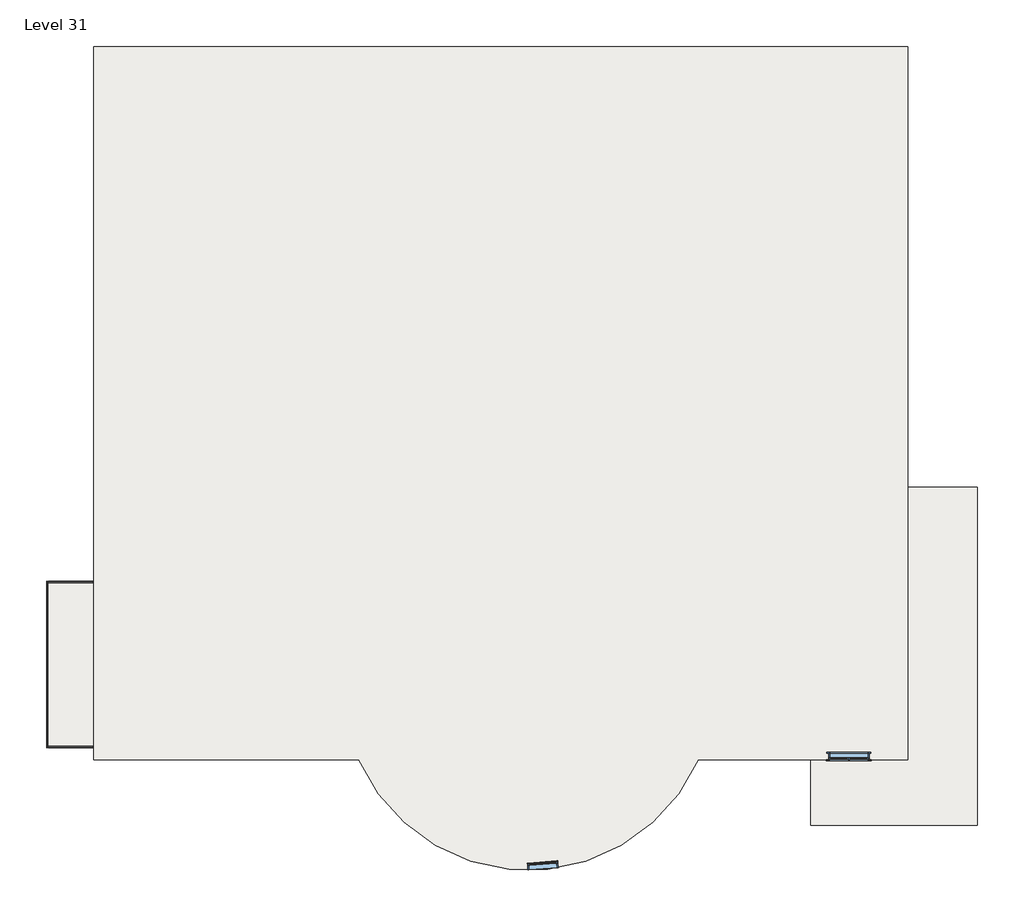
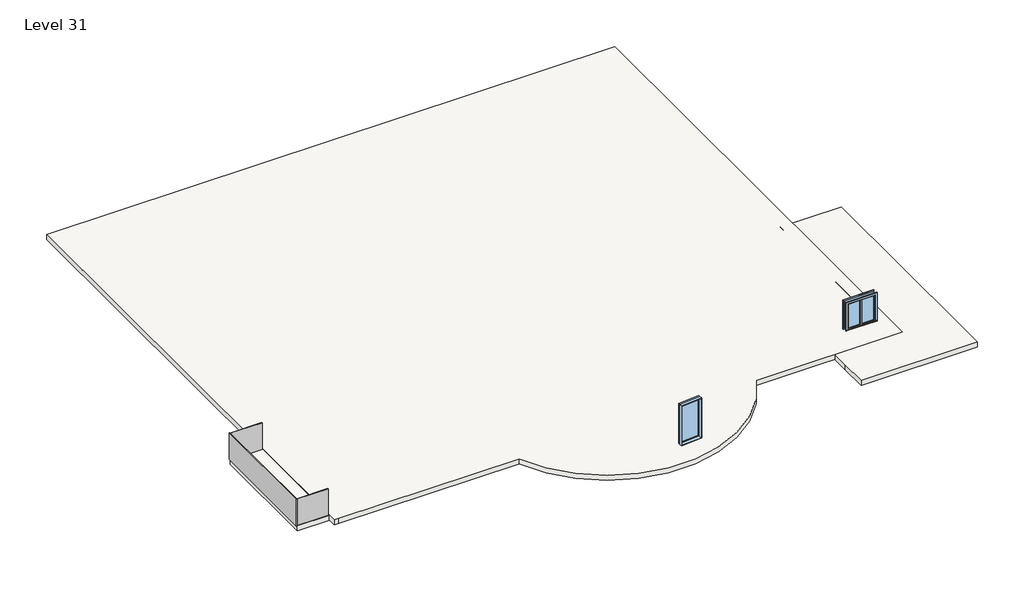
# One storey: 3 plates, 3 slabs, 2 windows.
"""IFC4 building model written with IfcOpenShell, lengths in millimetres."""

from ifc_helpers import new_model, si_unit, point, frame, frame_2d, origin, place, context, project, spatial, polyline, circle_curve, trimmed, segment, composite_curve, outline, extrude, transform, mapped, element, save
from components import system_panel_glazed_7d767388, system_panel_glazed_48506e1c, window_0862ab64, window_9a779fa2

model = new_model("IFC4")

# Units and contexts
model_context = context("Model", 3, world=origin())
ifc_project = project(units=[si_unit("LENGTHUNIT", "METRE", prefix="MILLI")], contexts=[model_context])

# Site, building, storey
site = spatial("IfcSite", under=ifc_project)
building = spatial("IfcBuilding", under=site)
storey = spatial("IfcBuildingStorey", under=building, Name="Level 31", Elevation=49149.0)

# Plates
placement = place(None, origin())
system_panel_glazed_shape = system_panel_glazed_7d767388(model_context)
element("IfcPlate", 1, ObjectType="System Panel : Glazed", at=placement, inside=storey, context=model_context, shape_type="MappedRepresentation", body=[
    mapped(system_panel_glazed_shape, transform((-17306.4505427, -8690.0239591, 49149.0), x_axis=(-1.0, 0.0, 0.0), y_axis=(0.0, -1.0, 0.0), z_axis=(0.0, 0.0, 1.0))),
])
element("IfcPlate", 2, ObjectType="System Panel : Glazed", at=placement, inside=storey, context=model_context, shape_type="MappedRepresentation", body=[
    mapped(system_panel_glazed_shape, transform((-17306.4505427, -13719.2239591, 49149.0), x_axis=(1.0, 0.0, 0.0), y_axis=(0.0, 1.0, 0.0), z_axis=(0.0, 0.0, 1.0))),
])
system_panel_glazed_2_shape = system_panel_glazed_48506e1c(model_context)
element("IfcPlate", 3, ObjectType="System Panel : Glazed", at=placement, inside=storey, context=model_context, shape_type="MappedRepresentation", body=[
    mapped(system_panel_glazed_2_shape, transform((-17979.5505427, -11204.6239591, 49149.0), x_axis=(0.0, -1.0, 0.0), y_axis=(1.0, 0.0, 0.0), z_axis=(0.0, 0.0, 1.0))),
])

# Slabs
element("IfcSlab", 4, ObjectType="9\"", at=placement, inside=storey, context=model_context, shape_type="SweptSolid", body=[
    extrude(outline(composite_curve([segment(polyline([(-16606.2882188, 7457.5128001), (7980.9117812, 7457.5128001), (7980.9117812, -14081.6871999), (1654.5363171, -14081.6871999)]), True, "CONTINUOUS"), segment(trimmed(circle_curve(frame_2d((-3474.4882188, -11791.9714001)), 5616.9111737), [point((1654.5363171, -14081.6871999))], [point((-8603.5127547, -14081.6871999))], False, "CARTESIAN"), True, "CONTINUOUS"), segment(polyline([(-8603.5127547, -14081.6871999), (-16403.0882188, -14081.6871999), (-16606.2882188, -14081.6871999), (-16606.2882188, 7457.5128001)]), True, "CONTINUOUS")], self_intersect=False)), frame((0.0, 0.0, 48926.9232641), z_axis=(0.0, 0.0, 1.0), x_axis=(1.0, 0.0, 0.0)), (0.0, 0.0, 1.0), 228.6),
])
element("IfcSlab", 5, ObjectType="9\"", at=placement, inside=storey, context=model_context, shape_type="SweptSolid", body=[
    extrude(outline(polyline([(-17978.526008, -8690.0239591), (-16606.926008, -8690.0239591), (-16606.926008, -13719.2239591), (-17978.526008, -13719.2239591), (-17978.526008, -8690.0239591)])), frame((0.0, 0.0, 48920.4), z_axis=(0.0, 0.0, 1.0), x_axis=(1.0, 0.0, 0.0)), (0.0, 0.0, 1.0), 228.6),
])
element("IfcSlab", 6, ObjectType="9\"", at=placement, inside=storey, context=model_context, shape_type="SweptSolid", body=[
    extrude(outline(polyline([(5053.3049901, -14840.0808221), (5053.3049901, -14078.0808221), (7237.7049901, -14078.0808221), (7440.9049901, -14078.0808221), (7440.9049901, -5848.4808221), (10082.5049901, -5848.4808221), (10082.5049901, -14840.0808221), (10082.5049901, -16059.2808221), (5053.3049901, -16059.2808221), (5053.3049901, -14840.0808221)])), frame((0.0, 0.0, 48920.4), z_axis=(0.0, 0.0, 1.0), x_axis=(1.0, 0.0, 0.0)), (0.0, 0.0, 1.0), 228.6),
])

# Windows
window_shape = window_0862ab64(model_context)
element("IfcWindow", 7, ObjectType="Casement Dbl with Trim : 48\" x 48\"", at=placement, inside=storey, context=model_context, shape_type="MappedRepresentation", body=[
    mapped(window_shape, transform((6201.2494573, -13957.4308221, 49149.0), x_axis=(-1.0, 0.0, 0.0), y_axis=(0.0, -1.0, 0.0), z_axis=(0.0, 0.0, 1.0))),
])
window_2_shape = window_9a779fa2(model_context)
element("IfcWindow", 8, ObjectType="Fixed : 36\" x 72\"", at=placement, inside=storey, context=model_context, shape_type="MappedRepresentation", body=[
    mapped(window_2_shape, transform((-3004.3436993, -17264.1796157, 49658.9372835), x_axis=(0.9968797467107341, 0.07893523039772918, 0.0), y_axis=(-0.07893523039772918, 0.9968797467107341, 0.0), z_axis=(0.0, 0.0, 1.0))),
])

save(model, "model.ifc")

# Revit data of these elements
# Type "System Panel : Glazed"
#   Construction Type Id = "GSP4R"
#   Analytic Construction = "1/8 in Pilkington single glazing"
#   Visual Light Transmittance = 0.9
#   Solar Heat Gain Coefficient = 0.86
#   Heat Transfer Coefficient (U) = 1.18115 BTU/(h·ft²·°F)
# Type "9\""
#   Assembly Code = "B1010"
#   Function = 0
#   Layers, outside or top first: 0' - 9" no material (function 1)
# Type "Casement Dbl with Trim : 48\" x 48\""
#   Type Mark = "10"
#   Construction Type Id = "GSP4R"
#   Assembly Code = "B2020100"
#   Analytic Construction = "1/8 in Pilkington single glazing"
#   Visual Light Transmittance = 0.9
#   Solar Heat Gain Coefficient = 0.78
#   Heat Transfer Coefficient (U) = 0.6496 BTU/(h·ft²·°F)
#   Height = 4' - 0"
#   Default Sill Height = 3' - 0"
#   Trim Projection - Ext. = 0' - 0 1/2"
#   Trim Projection - Int. = 0' - 0 3/4"
#   Trim Width - Exterior = 0' - 3 1/2"
#   Trim Width - Interior = 0' - 3 1/2"
#   Width = 4' - 0"
#   Window Inset = 0' - 0 3/4"
#   Define Thermal Properties by = 1
#   Glass Pane Material = Glass
#   Sash Material = Sash
#   Trim Exterior Material = Trim
#   Trim Interior Material = Trim
#   Wall Closure = (empty or 0)
# Type "Fixed : 36\" x 72\""
#   Type Mark = "9"
#   Construction Type Id = "GSP4R"
#   Assembly Code = "B2020100"
#   Analytic Construction = "1/8 in Pilkington single glazing"
#   Visual Light Transmittance = 0.9
#   Solar Heat Gain Coefficient = 0.78
#   Heat Transfer Coefficient (U) = 0.6496 BTU/(h·ft²·°F)
#   Height = 6' - 0"
#   Default Sill Height = 1' - 0"
#   Width = 3' - 0"
#   Window Inset = 0' - 0 3/4"
#   Define Thermal Properties by = 1
#   Glass Pane Material = Glass
#   Sash Material = Sash
#   Wall Closure = (empty or 0)
# Elements 1, 2, 3 (IfcPlate, "System Panel : Glazed")
#   Phase Created = New Construction
#   Materials on its faces: "Glass"
# Element 4 (IfcSlab, "9\"")
#   built-in parameter 1001955 = 1.5708 (stored number, unit not read)
#   Height Offset From Level = 0' - 0.25682"
#   Phase Created = New Construction
#   Materials on its faces: "Default Floor"
# Element 5 (IfcSlab, "9\"")
#   built-in parameter 1001955 = 3.14159 (stored number, unit not read)
#   Height Offset From Level = 0' - 0"
#   Phase Created = New Construction
#   Materials on its faces: "Default Floor"
# Element 6 (IfcSlab, "9\"")
#   built-in parameter 1001955 = -1.5708 (stored number, unit not read)
#   Height Offset From Level = 0' - 0"
#   Phase Created = New Construction
#   Materials on its faces: "Default Floor"
# Element 7 (IfcWindow, "Casement Dbl with Trim : 48\" x 48\"")
#   Mark = "46"
#   Phase Created = New Construction
#   Materials on its faces: "Sash", "Trim", "Glass"
# Element 8 (IfcWindow, "Fixed : 36\" x 72\"")
#   Mark = "1"
#   Phase Created = New Construction
#   Materials on its faces: "Sash", "Glass"
# Materials
#   "Glass": class "Glass", colour RGB 0 128 192, transparency 0.75, Description = "Soda Lime Glass", Cost = 0
#   "Sash": class "Wood", colour RGB 224 178 126, transparency 0
#   "Trim": class "Wood", colour RGB 224 178 126, transparency 0
#   "Default Floor": colour RGB 128 128 128, transparency 0
